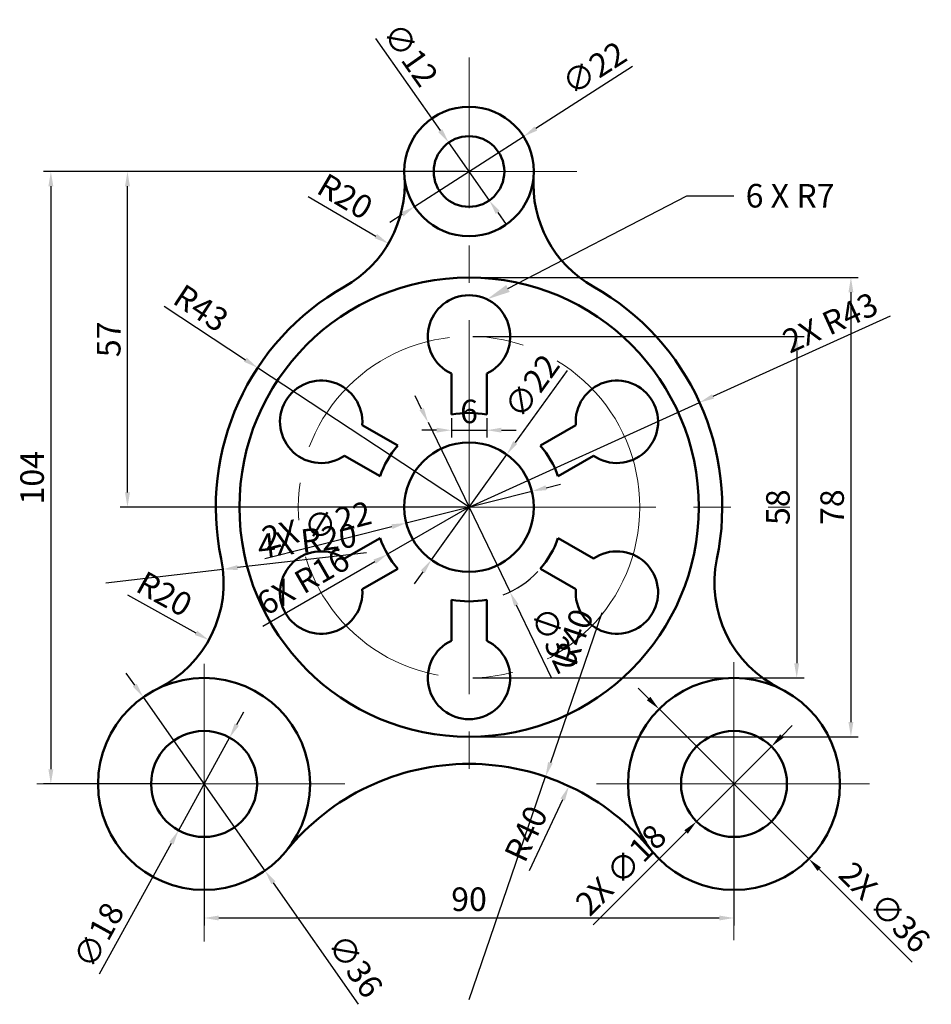
# Model space of a CAD drawing. Units: millimetres. Extents: x 3419 to 3574, y 1630 to 1797.
import ezdxf
from ezdxf import colors
from ezdxf.entities.mleader import LeaderData, LeaderLine
from ezdxf.math import Vec2, Vec3

# ---------------------------------------------------------------- set-up
doc = ezdxf.new("R2010")
doc.units = ezdxf.units.MM
doc.linetypes.add('CENTER', pattern=[50.8, 31.75, -6.35, 6.35, -6.35])
for name, color, linetype, lineweight in [('M-CNTR', 1, 'CENTER', 18), ('M-DIMS', 120, 'Continuous', 25), ('M-OUTL', 7, 'Continuous', 50)]:
    doc.layers.add(name, color=color, linetype=linetype, lineweight=lineweight)
doc.styles.get("Standard").update_dxf_attribs({"font": 'arial.ttf'})
doc.dimstyles.new('ISO-25', dxfattribs={"dimtxt": 4, "dimasz": 2.5, "dimexe": 1.25, "dimexo": 0.625, "dimtad": 1, "dimtxsty": 'Standard', "dimcen": 2.5, "dimadec": 0, "dimazin": 0, "dimtfac": 1, "dimtmove": 0, "dimatfit": 3, "dimfxl": 1, "dimarcsym": 0})

# ---------------------------------------------------------------- blocks, each defined once
blk = doc.blocks.new('*D1')
at = {"layer": 'Defpoints', "color": 0, "transparency": 16777216}
for p in [(3437.35, 1771.64), (3495.36, 1771.64), (3495.36, 1714.64)]:
    blk.add_point(p, dxfattribs=at)
at = {"layer": 'M-DIMS', "color": 0, "lineweight": -2, "transparency": 16777216}
for p, q in [((3494.74, 1771.64), (3436.1, 1771.64)), ((3437.35, 1717.14), (3437.35, 1769.14)), ((3494.74, 1714.64), (3436.1, 1714.64))]:
    blk.add_line(p, q, dxfattribs=at)
at = {"layer": 'M-DIMS', "color": 0, "transparency": 16777216}
for points in [[(3436.94, 1769.14), (3437.77, 1769.14), (3437.35, 1771.64)], [(3436.94, 1717.14), (3437.77, 1717.14), (3437.35, 1714.64)]]:
    blk.add_solid(points, dxfattribs=at)
at = {"layer": 'M-DIMS', "color": 0, "transparency": 16777216, "insert": (3434.69, 1743.14), "char_height": 4, "attachment_point": 5, "rotation": 90}
blk.add_mtext('57', dxfattribs=at)
blk = doc.blocks.new('*D2')
at = {"layer": 'Defpoints', "color": 0, "transparency": 16777216}
for p in [(3495.36, 1771.64), (3424.34, 1667.64), (3450.36, 1667.64)]:
    blk.add_point(p, dxfattribs=at)
at = {"layer": 'M-DIMS', "color": 0, "lineweight": -2, "transparency": 16777216}
for p, q in [((3494.74, 1771.64), (3423.09, 1771.64)), ((3424.34, 1769.14), (3424.34, 1670.14)), ((3449.74, 1667.64), (3423.09, 1667.64))]:
    blk.add_line(p, q, dxfattribs=at)
at = {"layer": 'M-DIMS', "color": 0, "transparency": 16777216}
for points in [[(3423.92, 1769.14), (3424.76, 1769.14), (3424.34, 1771.64)], [(3423.92, 1670.14), (3424.76, 1670.14), (3424.34, 1667.64)]]:
    blk.add_solid(points, dxfattribs=at)
at = {"layer": 'M-DIMS', "color": 0, "transparency": 16777216, "insert": (3421.67, 1719.64), "char_height": 4, "attachment_point": 5, "rotation": 90}
blk.add_mtext('104', dxfattribs=at)
blk = doc.blocks.new('*D3')
at = {"layer": 'Defpoints', "color": 0, "transparency": 16777216}
for p in [(3495.36, 1743.64), (3495.36, 1685.64), (3551.01, 1685.64)]:
    blk.add_point(p, dxfattribs=at)
at = {"layer": 'M-DIMS', "color": 0, "lineweight": -2, "transparency": 16777216}
for p, q in [((3495.99, 1743.64), (3552.26, 1743.64)), ((3551.01, 1741.14), (3551.01, 1688.14)), ((3495.99, 1685.64), (3552.26, 1685.64))]:
    blk.add_line(p, q, dxfattribs=at)
at = {"layer": 'M-DIMS', "color": 0, "transparency": 16777216}
for points in [[(3550.59, 1741.14), (3551.43, 1741.14), (3551.01, 1743.64)], [(3550.59, 1688.14), (3551.43, 1688.14), (3551.01, 1685.64)]]:
    blk.add_solid(points, dxfattribs=at)
at = {"layer": 'M-DIMS', "color": 0, "transparency": 16777216, "insert": (3548.34, 1714.64), "char_height": 4, "attachment_point": 5, "rotation": 90}
blk.add_mtext('58', dxfattribs=at)
blk = doc.blocks.new('*D4')
at = {"layer": 'Defpoints', "color": 0, "transparency": 16777216}
for p in [(3495.36, 1753.64), (3495.36, 1675.64), (3560.22, 1675.64)]:
    blk.add_point(p, dxfattribs=at)
at = {"layer": 'M-DIMS', "color": 0, "lineweight": -2, "transparency": 16777216}
for p, q in [((3495.99, 1753.64), (3561.47, 1753.64)), ((3560.22, 1751.14), (3560.22, 1678.14)), ((3495.99, 1675.64), (3561.47, 1675.64))]:
    blk.add_line(p, q, dxfattribs=at)
at = {"layer": 'M-DIMS', "color": 0, "transparency": 16777216}
for points in [[(3559.8, 1751.14), (3560.63, 1751.14), (3560.22, 1753.64)], [(3559.8, 1678.14), (3560.63, 1678.14), (3560.22, 1675.64)]]:
    blk.add_solid(points, dxfattribs=at)
at = {"layer": 'M-DIMS', "color": 0, "transparency": 16777216, "insert": (3557.55, 1714.64), "char_height": 4, "attachment_point": 5, "rotation": 90}
blk.add_mtext('78', dxfattribs=at)
blk = doc.blocks.new('*D5')
at = {"layer": 'Defpoints', "color": 0, "transparency": 16777216}
for p in [(3450.36, 1667.64), (3540.36, 1667.64), (3540.36, 1644.88)]:
    blk.add_point(p, dxfattribs=at)
at = {"layer": 'M-DIMS', "color": 0, "lineweight": -2, "transparency": 16777216}
for p, q in [((3450.36, 1667.01), (3450.36, 1643.63)), ((3540.36, 1667.01), (3540.36, 1643.63)), ((3452.86, 1644.88), (3537.86, 1644.88))]:
    blk.add_line(p, q, dxfattribs=at)
at = {"layer": 'M-DIMS', "color": 0, "transparency": 16777216}
for points in [[(3452.86, 1645.3), (3452.86, 1644.46), (3450.36, 1644.88)], [(3537.86, 1645.3), (3537.86, 1644.46), (3540.36, 1644.88)]]:
    blk.add_solid(points, dxfattribs=at)
at = {"layer": 'M-DIMS', "color": 0, "transparency": 16777216, "insert": (3495.36, 1647.55), "char_height": 4, "attachment_point": 5}
blk.add_mtext('90', dxfattribs=at)
blk = doc.blocks.new('*D6')
at = {"layer": 'Defpoints', "color": 0, "transparency": 16777216}
for p in [(3464.43, 1769.53), (3481.68, 1759.4)]:
    blk.add_point(p, dxfattribs=at)
at = {"layer": 'M-DIMS', "color": 0, "lineweight": -2, "transparency": 16777216}
blk.add_line((3468.06, 1767.4), (3479.53, 1760.67), dxfattribs=at)
at = {"layer": 'M-DIMS', "color": 0, "transparency": 16777216}
blk.add_solid([(3479.74, 1761.03), (3479.32, 1760.31), (3481.68, 1759.4)], dxfattribs=at)
at = {"layer": 'M-DIMS', "color": 0, "transparency": 16777216, "insert": (3474.06, 1766.97), "char_height": 4, "attachment_point": 5, "rotation": 329.5958}
blk.add_mtext('R20', dxfattribs=at)
blk = doc.blocks.new('*D7')
at = {"layer": 'Defpoints', "color": 0, "transparency": 16777216}
for p in [(3512.34, 1667.27), (3495.36, 1631.05)]:
    blk.add_point(p, dxfattribs=at)
at = {"layer": 'M-DIMS', "color": 0, "lineweight": -2, "transparency": 16777216}
blk.add_line((3505.63, 1652.96), (3511.28, 1665), dxfattribs=at)
at = {"layer": 'M-DIMS', "color": 0, "transparency": 16777216}
blk.add_solid([(3510.9, 1665.18), (3511.65, 1664.82), (3512.34, 1667.27)], dxfattribs=at)
at = {"layer": 'M-DIMS', "color": 0, "transparency": 16777216, "insert": (3505.51, 1658.98), "char_height": 4, "attachment_point": 5, "rotation": 64.8845}
blk.add_mtext('R40', dxfattribs=at)
blk = doc.blocks.new('*D8')
at = {"layer": 'Defpoints', "color": 0, "transparency": 16777216}
for p in [(3433.69, 1701.79), (3451.17, 1692.08)]:
    blk.add_point(p, dxfattribs=at)
at = {"layer": 'M-DIMS', "color": 0, "lineweight": -2, "transparency": 16777216}
blk.add_line((3437.36, 1699.75), (3448.99, 1693.29), dxfattribs=at)
at = {"layer": 'M-DIMS', "color": 0, "transparency": 16777216}
blk.add_solid([(3449.19, 1693.66), (3448.79, 1692.93), (3451.17, 1692.08)], dxfattribs=at)
at = {"layer": 'M-DIMS', "color": 0, "transparency": 16777216, "insert": (3443.38, 1699.46), "char_height": 4, "attachment_point": 5, "rotation": 330.9757}
blk.add_mtext('R20', dxfattribs=at)
blk = doc.blocks.new('*D9')
at = {"layer": 'Defpoints', "color": 0, "transparency": 16777216}
for p in [(3459.46, 1738.31), (3495.36, 1714.64)]:
    blk.add_point(p, dxfattribs=at)
at = {"layer": 'M-DIMS', "color": 0, "lineweight": -2, "transparency": 16777216}
for p, q in [((3443.59, 1748.77), (3457.37, 1739.68)), ((3495.36, 1714.64), (3459.46, 1738.31))]:
    blk.add_line(p, q, dxfattribs=at)
at = {"layer": 'M-DIMS', "color": 0, "transparency": 16777216}
blk.add_solid([(3457.6, 1740.03), (3457.14, 1739.33), (3459.46, 1738.31)], dxfattribs=at)
at = {"layer": 'M-DIMS', "color": 0, "transparency": 16777216, "insert": (3449.57, 1748.02), "char_height": 4, "attachment_point": 5, "rotation": 326.6072}
blk.add_mtext('R43', dxfattribs=at)
blk = doc.blocks.new('*D10')
at = {"layer": 'Defpoints', "color": 0, "transparency": 16777216}
for p in [(3504.62, 1777.58), (3486.11, 1765.69)]:
    blk.add_point(p, dxfattribs=at)
at = {"layer": 'M-DIMS', "color": 0, "lineweight": -2, "transparency": 16777216}
for p, q in [((3523.15, 1789.49), (3506.72, 1778.94)), ((3486.11, 1765.69), (3504.62, 1777.58)), ((3484, 1764.34), (3481.9, 1762.99))]:
    blk.add_line(p, q, dxfattribs=at)
at = {"layer": 'M-DIMS', "color": 0, "transparency": 16777216}
for points in [[(3506.49, 1779.29), (3506.94, 1778.59), (3504.62, 1777.58)], [(3483.78, 1764.69), (3484.23, 1763.99), (3486.11, 1765.69)]]:
    blk.add_solid(points, dxfattribs=at)
at = {"layer": 'M-DIMS', "color": 0, "transparency": 16777216, "insert": (3516.89, 1788.77), "char_height": 4, "attachment_point": 5, "rotation": 32.7148}
blk.add_mtext('∅22', dxfattribs=at)
blk = doc.blocks.new('*D11')
at = {"layer": 'Defpoints', "color": 0, "transparency": 16777216}
for p in [(3491.91, 1776.55), (3498.81, 1766.73)]:
    blk.add_point(p, dxfattribs=at)
at = {"layer": 'M-DIMS', "color": 0, "lineweight": -2, "transparency": 16777216}
for p, q in [((3479.5, 1794.22), (3490.48, 1778.6)), ((3498.81, 1766.73), (3491.91, 1776.55)), ((3500.25, 1764.68), (3501.68, 1762.64))]:
    blk.add_line(p, q, dxfattribs=at)
at = {"layer": 'M-DIMS', "color": 0, "transparency": 16777216}
for points in [[(3490.82, 1778.83), (3490.13, 1778.36), (3491.91, 1776.55)], [(3500.59, 1764.92), (3499.9, 1764.44), (3498.81, 1766.73)]]:
    blk.add_solid(points, dxfattribs=at)
at = {"layer": 'M-DIMS', "color": 0, "transparency": 16777216, "insert": (3485.02, 1791.2), "char_height": 4, "attachment_point": 5, "rotation": 305.0799}
blk.add_mtext('∅12', dxfattribs=at)
blk = doc.blocks.new('*D12')
at = {"layer": 'Defpoints', "color": 0, "transparency": 16777216}
for p in [(3440.02, 1682.38), (3460.7, 1652.9)]:
    blk.add_point(p, dxfattribs=at)
at = {"layer": 'M-DIMS', "color": 0, "lineweight": -2, "transparency": 16777216}
for p, q in [((3438.59, 1684.42), (3437.15, 1686.47)), ((3440.02, 1682.38), (3460.7, 1652.9)), ((3476.6, 1630.22), (3462.13, 1650.86))]:
    blk.add_line(p, q, dxfattribs=at)
at = {"layer": 'M-DIMS', "color": 0, "transparency": 16777216}
for points in [[(3438.93, 1684.66), (3438.25, 1684.18), (3440.02, 1682.38)], [(3462.47, 1651.1), (3461.79, 1650.62), (3460.7, 1652.9)]]:
    blk.add_solid(points, dxfattribs=at)
at = {"layer": 'M-DIMS', "color": 0, "transparency": 16777216, "insert": (3475.63, 1636.46), "char_height": 4, "attachment_point": 5, "rotation": 305.0463}
blk.add_mtext('∅36', dxfattribs=at)
blk = doc.blocks.new('*D13')
at = {"layer": 'Defpoints', "color": 0, "transparency": 16777216}
for p in [(3454.7, 1675.52), (3446.02, 1659.76)]:
    blk.add_point(p, dxfattribs=at)
at = {"layer": 'M-DIMS', "color": 0, "lineweight": -2, "transparency": 16777216}
for p, q in [((3455.91, 1677.71), (3457.12, 1679.9)), ((3454.7, 1675.52), (3446.02, 1659.76)), ((3432.59, 1635.4), (3444.81, 1657.57))]:
    blk.add_line(p, q, dxfattribs=at)
at = {"layer": 'M-DIMS', "color": 0, "transparency": 16777216}
for points in [[(3455.55, 1677.91), (3456.28, 1677.51), (3454.7, 1675.52)], [(3444.45, 1657.77), (3445.18, 1657.37), (3446.02, 1659.76)]]:
    blk.add_solid(points, dxfattribs=at)
at = {"layer": 'M-DIMS', "color": 0, "transparency": 16777216, "insert": (3432.9, 1641.7), "char_height": 4, "attachment_point": 5, "rotation": 61.1443}
blk.add_mtext('∅18', dxfattribs=at)
blk = doc.blocks.new('*D14')
at = {"layer": 'Defpoints', "color": 0, "transparency": 16777216}
for p in [(3501.77, 1723.58), (3488.96, 1705.7)]:
    blk.add_point(p, dxfattribs=at)
at = {"layer": 'M-DIMS', "color": 0, "lineweight": -2, "transparency": 16777216}
for p, q in [((3512, 1737.87), (3503.22, 1725.61)), ((3488.96, 1705.7), (3501.77, 1723.58)), ((3487.5, 1703.66), (3486.04, 1701.63))]:
    blk.add_line(p, q, dxfattribs=at)
at = {"layer": 'M-DIMS', "color": 0, "transparency": 16777216}
for points in [[(3502.88, 1725.86), (3503.56, 1725.37), (3501.77, 1723.58)], [(3487.16, 1703.91), (3487.84, 1703.42), (3488.96, 1705.7)]]:
    blk.add_solid(points, dxfattribs=at)
at = {"layer": 'M-DIMS', "color": 0, "transparency": 16777216, "insert": (3506.45, 1734.89), "char_height": 4, "attachment_point": 5, "rotation": 54.389}
blk.add_mtext('∅22', dxfattribs=at)
blk = doc.blocks.new('*D15')
at = {"layer": 'Defpoints', "color": 0, "transparency": 16777216}
for p in [(3488.4, 1729.05), (3502.32, 1700.23)]:
    blk.add_point(p, dxfattribs=at)
at = {"layer": 'M-DIMS', "color": 0, "lineweight": -2, "transparency": 16777216}
for p, q in [((3487.31, 1731.3), (3486.22, 1733.55)), ((3488.4, 1729.05), (3502.32, 1700.23)), ((3509.41, 1685.56), (3503.41, 1697.98))]:
    blk.add_line(p, q, dxfattribs=at)
blk.add_arc((3495.36, 1714.64), 16, 291.3129, 316.955, dxfattribs=at)
at = {"layer": 'M-DIMS', "color": 0, "transparency": 16777216}
for points in [[(3487.69, 1731.48), (3486.94, 1731.12), (3488.4, 1729.05)], [(3503.78, 1698.16), (3503.03, 1697.8), (3502.32, 1700.23)]]:
    blk.add_solid(points, dxfattribs=at)
at = {"layer": 'M-DIMS', "color": 0, "transparency": 16777216, "insert": (3509.46, 1691.86), "char_height": 4, "attachment_point": 5, "rotation": 295.7891}
blk.add_mtext('∅32', dxfattribs=at)
blk = doc.blocks.new('*D16')
at = {"layer": 'Defpoints', "color": 0, "transparency": 16777216}
for p in [(3492.36, 1730.36), (3498.36, 1730.36), (3498.36, 1727.71)]:
    blk.add_point(p, dxfattribs=at)
at = {"layer": 'M-DIMS', "color": 0, "lineweight": -2, "transparency": 16777216}
for p, q in [((3492.36, 1729.73), (3492.36, 1726.46)), ((3498.36, 1729.73), (3498.36, 1726.46)), ((3489.86, 1727.71), (3487.36, 1727.71)), ((3492.36, 1727.71), (3498.36, 1727.71)), ((3500.86, 1727.71), (3503.36, 1727.71))]:
    blk.add_line(p, q, dxfattribs=at)
at = {"layer": 'M-DIMS', "color": 0, "transparency": 16777216}
for points in [[(3489.86, 1728.13), (3489.86, 1727.3), (3492.36, 1727.71)], [(3500.86, 1728.13), (3500.86, 1727.3), (3498.36, 1727.71)]]:
    blk.add_solid(points, dxfattribs=at)
at = {"layer": 'M-DIMS', "color": 0, "transparency": 16777216, "insert": (3495.36, 1730.38), "char_height": 4, "attachment_point": 5}
blk.add_mtext('6', dxfattribs=at)
blk = doc.blocks.new('KEYHOLE-D14-W6')
for p, q in [((4, 6.96), (4, 0)), ((10, 6.96), (10, 0))]:
    blk.add_line(p, q)
for centre, radius, start, end in [((7, 13.28), 7, 295.3769, 244.6231), ((7, -15.72), 16, 79.1931, 100.8069)]:
    blk.add_arc(centre, radius, start, end)
blk = doc.blocks.new('MOUNTING-BOSS-D36-D18')
for radius in [18, 9]:
    blk.add_circle((18, 18), radius)
blk = doc.blocks.new('*D19')
at = {"layer": 'Defpoints', "color": 0, "transparency": 16777216}
for p in [(3534.52, 1732.41), (3495.36, 1714.64)]:
    blk.add_point(p, dxfattribs=at)
at = {"layer": 'M-DIMS', "color": 0, "lineweight": -2, "transparency": 16777216}
for p, q in [((3566.87, 1747.1), (3536.79, 1733.45)), ((3495.36, 1714.64), (3534.52, 1732.41))]:
    blk.add_line(p, q, dxfattribs=at)
at = {"layer": 'M-DIMS', "color": 0, "transparency": 16777216}
blk.add_solid([(3536.62, 1733.82), (3536.96, 1733.07), (3534.52, 1732.41)], dxfattribs=at)
at = {"layer": 'M-DIMS', "color": 0, "transparency": 16777216, "insert": (3556.91, 1745.51), "char_height": 4, "attachment_point": 5, "rotation": 24.413}
blk.add_mtext('2X R43', dxfattribs=at)
blk = doc.blocks.new('*D20')
at = {"layer": 'Defpoints', "color": 0, "transparency": 16777216}
for p in [(3506.03, 1717.33), (3484.69, 1711.95)]:
    blk.add_point(p, dxfattribs=at)
at = {"layer": 'M-DIMS', "color": 0, "lineweight": -2, "transparency": 16777216}
for p, q in [((3506.03, 1717.33), (3484.69, 1711.95)), ((3508.45, 1717.94), (3510.88, 1718.55)), ((3460.7, 1705.9), (3482.27, 1711.34))]:
    blk.add_line(p, q, dxfattribs=at)
at = {"layer": 'M-DIMS', "color": 0, "transparency": 16777216}
for points in [[(3508.35, 1718.34), (3508.55, 1717.54), (3506.03, 1717.33)], [(3482.17, 1711.74), (3482.37, 1710.94), (3484.69, 1711.95)]]:
    blk.add_solid(points, dxfattribs=at)
at = {"layer": 'M-DIMS', "color": 0, "transparency": 16777216, "insert": (3469.6, 1711.01), "char_height": 4, "attachment_point": 5, "rotation": 14.1494}
blk.add_mtext('2X ∅22', dxfattribs=at)
blk = doc.blocks.new('*D21')
at = {"layer": 'Defpoints', "color": 0, "transparency": 16777216}
for p in [(3453.55, 1704.09), (3433.69, 1701.79)]:
    blk.add_point(p, dxfattribs=at)
at = {"layer": 'M-DIMS', "color": 0, "lineweight": -2, "transparency": 16777216}
for p, q in [((3477.94, 1706.91), (3456.04, 1704.37)), ((3433.69, 1701.79), (3453.55, 1704.09))]:
    blk.add_line(p, q, dxfattribs=at)
at = {"layer": 'M-DIMS', "color": 0, "transparency": 16777216}
blk.add_solid([(3455.99, 1704.79), (3456.08, 1703.96), (3453.55, 1704.09)], dxfattribs=at)
at = {"layer": 'M-DIMS', "color": 0, "transparency": 16777216, "insert": (3467.92, 1708.44), "char_height": 4, "attachment_point": 5, "rotation": 6.6057}
blk.add_mtext('4X R20', dxfattribs=at)
blk = doc.blocks.new('*D22')
at = {"layer": 'Defpoints', "color": 0, "transparency": 16777216}
for p in [(3527.63, 1680.37), (3553.09, 1654.91)]:
    blk.add_point(p, dxfattribs=at)
at = {"layer": 'M-DIMS', "color": 0, "lineweight": -2, "transparency": 16777216}
for p, q in [((3525.86, 1682.13), (3524.1, 1683.9)), ((3527.63, 1680.37), (3553.09, 1654.91)), ((3570.61, 1637.39), (3554.86, 1653.14))]:
    blk.add_line(p, q, dxfattribs=at)
at = {"layer": 'M-DIMS', "color": 0, "transparency": 16777216}
for points in [[(3526.16, 1682.43), (3525.57, 1681.84), (3527.63, 1680.37)], [(3555.15, 1653.44), (3554.56, 1652.85), (3553.09, 1654.91)]]:
    blk.add_solid(points, dxfattribs=at)
at = {"layer": 'M-DIMS', "color": 0, "transparency": 16777216, "insert": (3565.58, 1646.35), "char_height": 4, "attachment_point": 5, "rotation": 315.0021}
blk.add_mtext('2X ∅36', dxfattribs=at)
blk = doc.blocks.new('*D23')
at = {"layer": 'Defpoints', "color": 0, "transparency": 16777216}
for p in [(3546.72, 1674.01), (3534, 1661.27)]:
    blk.add_point(p, dxfattribs=at)
at = {"layer": 'M-DIMS', "color": 0, "lineweight": -2, "transparency": 16777216}
for p, q in [((3548.49, 1675.77), (3550.26, 1677.54)), ((3546.72, 1674.01), (3534, 1661.27)), ((3516.47, 1643.74), (3532.23, 1659.51))]:
    blk.add_line(p, q, dxfattribs=at)
at = {"layer": 'M-DIMS', "color": 0, "transparency": 16777216}
for points in [[(3548.2, 1676.07), (3548.79, 1675.48), (3546.72, 1674.01)], [(3531.94, 1659.8), (3532.53, 1659.21), (3534, 1661.27)]]:
    blk.add_solid(points, dxfattribs=at)
at = {"layer": 'M-DIMS', "color": 0, "transparency": 16777216, "insert": (3521.5, 1652.7), "char_height": 4, "attachment_point": 5, "rotation": 45.0136}
blk.add_mtext('2X ∅18', dxfattribs=at)
blk = doc.blocks.new('*D24')
at = {"layer": 'Defpoints', "color": 0, "transparency": 16777216}
for p in [(3495.36, 1714.64), (3481.5, 1706.64)]:
    blk.add_point(p, dxfattribs=at)
at = {"layer": 'M-DIMS', "color": 0, "lineweight": -2, "transparency": 16777216}
for p, q in [((3495.36, 1714.64), (3481.5, 1706.64)), ((3460.35, 1694.43), (3479.34, 1705.39))]:
    blk.add_line(p, q, dxfattribs=at)
at = {"layer": 'M-DIMS', "color": 0, "transparency": 16777216}
blk.add_solid([(3479.13, 1705.75), (3479.55, 1705.03), (3481.5, 1706.64)], dxfattribs=at)
at = {"layer": 'M-DIMS', "color": 0, "transparency": 16777216, "insert": (3467.43, 1701.59), "char_height": 4, "attachment_point": 5, "rotation": 29.9984}
blk.add_mtext('6X R16', dxfattribs=at)
blk = doc.blocks.new('*D25')
at = {"layer": 'Defpoints', "color": 0, "transparency": 16777216}
for p in [(3508.36, 1668.88), (3495.36, 1631.05)]:
    blk.add_point(p, dxfattribs=at)
at = {"layer": 'M-DIMS', "color": 0, "lineweight": -2, "transparency": 16777216}
for p, q in [((3517.91, 1696.68), (3509.17, 1671.24)), ((3495.36, 1631.05), (3508.36, 1668.88))]:
    blk.add_line(p, q, dxfattribs=at)
at = {"layer": 'M-DIMS', "color": 0, "transparency": 16777216}
blk.add_solid([(3508.78, 1671.38), (3509.57, 1671.11), (3508.36, 1668.88)], dxfattribs=at)
at = {"layer": 'M-DIMS', "color": 0, "transparency": 16777216, "insert": (3513.64, 1692.44), "char_height": 4, "attachment_point": 5, "rotation": 71.0366}
blk.add_mtext('R40', dxfattribs=at)

msp = doc.modelspace()

# ---------------------------------------------------------------- linework, layer by layer
at = {"layer": 'M-CNTR'}
for p, q in [((3495.361, 1771.64), (3495.361, 1791.009)), ((3495.361, 1771.64), (3477.223, 1771.64)), ((3495.361, 1714.64), (3495.361, 1771.64)), ((3495.361, 1771.64), (3513.682, 1771.64)), ((3495.361, 1714.64), (3441.681, 1714.64)), ((3495.361, 1714.64), (3495.361, 1667.64)), ((3495.361, 1714.64), (3549.823, 1714.64)), ((3450.361, 1667.64), (3450.361, 1688.054)), ((3540.361, 1667.64), (3540.361, 1688.348)), ((3450.361, 1667.64), (3421.967, 1667.64)), ((3450.361, 1667.64), (3474.278, 1667.64)), ((3450.361, 1667.64), (3450.361, 1640.885)), ((3540.361, 1667.64), (3516.996, 1667.64)), ((3540.361, 1667.64), (3540.361, 1641.122)), ((3540.361, 1667.64), (3563.402, 1667.64))]:
    msp.add_line(p, q, dxfattribs=at)
msp.add_circle((3495.361, 1714.64), 29, dxfattribs=at)
at = {"layer": 'M-OUTL'}
for centre, radius in [((3495.361, 1771.64), 11), ((3495.361, 1771.64), 6), ((3495.361, 1714.64), 39), ((3495.361, 1714.64), 11)]:
    msp.add_circle(centre, radius, dxfattribs=at)
for centre, radius, start, end in [((3464.433, 1769.525), 20, 299.40094, 3.9103), ((3526.288, 1769.525), 20, 176.0897, 240.59906), ((3495.361, 1714.64), 43, 119.40094, 191.77278), ((3495.361, 1714.64), 43, 348.22722, 60.59906), ((3433.686, 1701.786), 20, 296.02794, 11.77278), ((3557.035, 1701.786), 20, 168.22722, 243.97206), ((3495.361, 1631.047), 40, 39.11674, 140.88326)]:
    msp.add_arc(centre, radius, start, end, dxfattribs=at)

# ---------------------------------------------------------------- block references
for name, p in [('KEYHOLE-D14-W6', (3488.36, 1730.356)), ('MOUNTING-BOSS-D36-D18', (3432.361, 1649.64)), ('MOUNTING-BOSS-D36-D18', (3522.361, 1649.64))]:
    msp.add_blockref(name, p, dxfattribs=at)
for p, rotation in [((3478.249, 1716.435), 59.99999999999529), ((3505.471, 1728.56), 299.999999999997), ((3485.25, 1700.719), 119.999999999997), ((3512.472, 1712.844), 240.0000000000009), ((3502.361, 1698.923), 180)]:
    msp.add_blockref('KEYHOLE-D14-W6', p, dxfattribs=dict(at, rotation=rotation))

# ---------------------------------------------------------------- dimensions: what is measured, and where the dimension line sits
at = {"layer": 'M-DIMS'}
for p1, p2, picture, middle in [((3498.809, 1766.729), (3491.912, 1776.55), '*D11', (3482.747, 1789.6)), ((3486.105, 1765.694), (3504.616, 1777.585), '*D10', (3518.396, 1786.437)), ((3488.955, 1705.697), (3501.766, 1723.582), '*D14', (3508.709, 1733.276)), ((3440.024, 1682.376), (3460.697, 1652.903), '*D12', (3473.351, 1634.862)), ((3454.704, 1675.522), (3446.017, 1659.757), '*D13', (3435.331, 1640.363))]:
    dim = msp.add_diameter_dim_2p(p1=p1, p2=p2, dimstyle='ISO-25', override={"dimclrd": 0, "dimclre": 0, "dimclrt": 0}, dxfattribs=at)
    dim.commit()
    dim.dimension.update_dxf_attribs({"geometry": picture, "text_midpoint": middle, "dimtype": 163})
for base, p1, p2, picture, middle in [((3424.339, 1667.64), (3495.361, 1771.64), (3450.361, 1667.64), '*D2', (3421.672, 1719.64)), ((3437.352, 1771.64), (3495.361, 1714.64), (3495.361, 1771.64), '*D1', (3434.693, 1743.14)), ((3560.216, 1675.64), (3495.361, 1753.64), (3495.361, 1675.64), '*D4', (3557.549, 1714.64)), ((3551.008, 1685.64), (3495.361, 1743.64), (3495.361, 1685.64), '*D3', (3548.341, 1714.64))]:
    dim = msp.add_linear_dim(base=base, p1=p1, p2=p2, angle=90, dimstyle='ISO-25', override={"dimclrd": 0, "dimclre": 0, "dimclrt": 0}, dxfattribs=at)
    dim.commit()
    dim.dimension.update_dxf_attribs({"geometry": picture, "text_midpoint": middle})
for center, mpoint, override, picture, middle in [((3464.433, 1769.525), (3481.682, 1759.404), {"dimclrd": 0, "dimclre": 0, "dimclrt": 0}, '*D6', (3472.715, 1764.666)), ((3495.361, 1714.64), (3459.459, 1738.306), {"dimclrd": 0, "dimclre": 0, "dimclrt": 0}, '*D9', (3448.098, 1745.795)), ((3433.686, 1701.786), (3451.174, 1692.082), {"dimclrd": 0, "dimclre": 0, "dimclrt": 0}, '*D8', (3442.083, 1697.126)), ((3495.361, 1631.047), (3508.359, 1668.876), {"dimdec": 0, "dimlfac": 1, "dimrnd": 0, "dimzin": 0, "dimdsep": 46, "dimlunit": 2}, '*D25', (3516.158, 1691.574)), ((3495.361, 1631.047), (3512.338, 1667.265), {"dimclrd": 0, "dimclre": 0, "dimclrt": 0}, '*D7', (3507.925, 1657.851))]:
    dim = msp.add_radius_dim(center=center, mpoint=mpoint, dimstyle='ISO-25', override=override, dxfattribs=at)
    dim.commit()
    dim.dimension.update_dxf_attribs({"geometry": picture, "text_midpoint": middle, "dimtype": 164})
dim = msp.add_radius_dim(center=(3495.361, 1714.64), mpoint=(3534.516, 1732.412), text='2X <>', dimstyle='ISO-25', override={"dimdec": 0, "dimlfac": 1, "dimrnd": 0, "dimzin": 0, "dimdsep": 46, "dimlunit": 2}, dxfattribs=at)
dim.commit()
dim.dimension.update_dxf_attribs({"geometry": '*D19', "text_midpoint": (3558.009, 1743.075), "dimtype": 164})
dim = msp.add_diameter_dim_2p(p1=(3488.4, 1729.046), p2=(3502.321, 1700.233), dimstyle='ISO-25', override={"dimclrd": 0, "dimclre": 0, "dimclrt": 0}, dxfattribs=at)
dim.commit()
dim.dimension.update_dxf_attribs({"geometry": '*D15', "text_midpoint": (3509.455, 1691.857)})
for base, p1, p2, picture, middle in [((3498.361, 1727.713), (3492.361, 1730.356), (3498.361, 1730.356), '*D16', (3495.361, 1730.381)), ((3540.361, 1644.88), (3450.361, 1667.64), (3540.361, 1667.64), '*D5', (3495.361, 1647.548))]:
    dim = msp.add_linear_dim(base=base, p1=p1, p2=p2, dimstyle='ISO-25', override={"dimclrd": 0, "dimclre": 0, "dimclrt": 0}, dxfattribs=at)
    dim.commit()
    dim.dimension.update_dxf_attribs({"geometry": picture, "text_midpoint": middle})
for p1, p2, picture, middle in [((3506.027, 1717.329), (3484.694, 1711.951), '*D20', (3470.275, 1708.315)), ((3546.723, 1674.005), (3533.998, 1661.274), '*D23', (3523.468, 1650.739))]:
    dim = msp.add_diameter_dim_2p(p1=p1, p2=p2, text='2X <>', dimstyle='ISO-25', override={"dimdec": 0, "dimlfac": 1, "dimrnd": 0, "dimzin": 0, "dimdsep": 46, "dimlunit": 2}, dxfattribs=at)
    dim.commit()
    dim.dimension.update_dxf_attribs({"geometry": picture, "text_midpoint": middle, "dimtype": 163})
for center, mpoint, text, picture, middle in [((3433.686, 1701.786), (3453.553, 1704.086), '4X <>', '*D21', (3467.923, 1708.436)), ((3495.361, 1714.64), (3481.504, 1706.64), '6X <>', '*D24', (3467.43, 1701.595))]:
    dim = msp.add_radius_dim(center=center, mpoint=mpoint, text=text, dimstyle='ISO-25', override={"dimdec": 0, "dimlfac": 1, "dimrnd": 0, "dimzin": 0, "dimdsep": 46, "dimlunit": 2}, dxfattribs=at)
    dim.commit()
    dim.dimension.update_dxf_attribs({"geometry": picture, "text_midpoint": middle})
dim = msp.add_diameter_dim_2p(p1=(3527.632, 1680.367), p2=(3553.089, 1654.912), text='2X <>', dimstyle='ISO-25', override={"dimdec": 0, "dimlfac": 1, "dimrnd": 0, "dimzin": 0, "dimdsep": 46, "dimlunit": 2}, dxfattribs=at)
dim.commit()
dim.dimension.update_dxf_attribs({"geometry": '*D22', "text_midpoint": (3563.618, 1644.384)})

# ---------------------------------------------------------------- leaders
ml = msp.add_multileader_mtext('Standard', dxfattribs=at)
ml.set_content('6 X R7', color=256)
ml.set_leader_properties()
ml.build(insert=Vec2(0, 0))
ctx = ml.context
ctx.base_point, ctx.plane_origin = Vec3(3540.343, 1767.491), Vec3(3498.416, 1749.938)
notes = []
notes.append((ctx, [(0, (1, 1, 0), (3532.343, 1767.491), (1, 0), 8, [(0, [(3498.416, 1749.938)], 0, [])])]))
ctx.mtext.insert, ctx.mtext.flow_direction = Vec3(3542.343, 1769.525), 5
for ctx, leaders in notes:
    for number, flags, end, landing, length, lines in leaders:
        leader = LeaderData()
        leader.index, (leader.has_last_leader_line, leader.has_dogleg_vector, leader.attachment_direction) = number, flags
        leader.last_leader_point, leader.dogleg_vector, leader.dogleg_length = Vec3(end), Vec3(landing), length
        for number, points, colour, breaks in lines:
            line = LeaderLine()
            line.index, line.vertices, line.color, line.breaks = number, Vec3.list(points), colors.encode_raw_color(colour), breaks
            leader.lines.append(line)
        ctx.leaders.append(leader)

doc.saveas('drawing.dxf')
